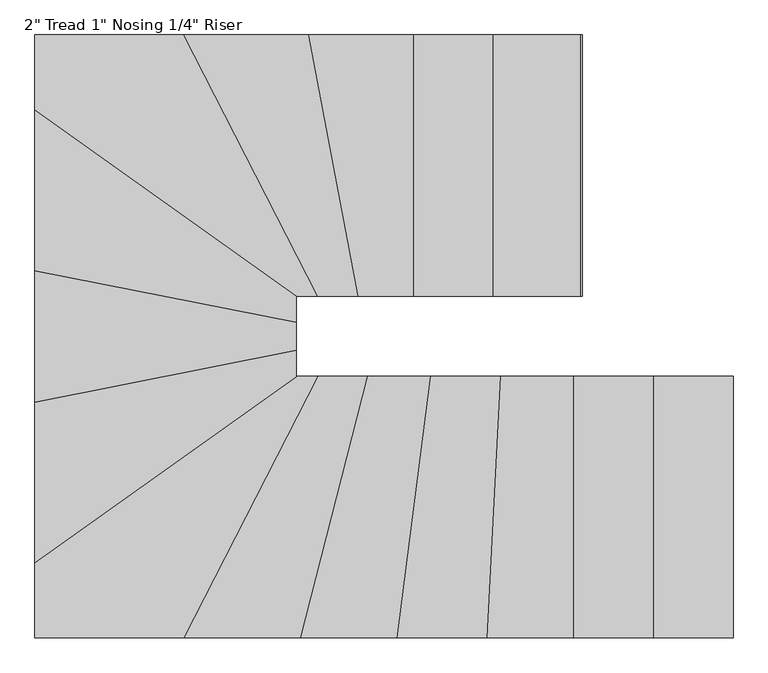
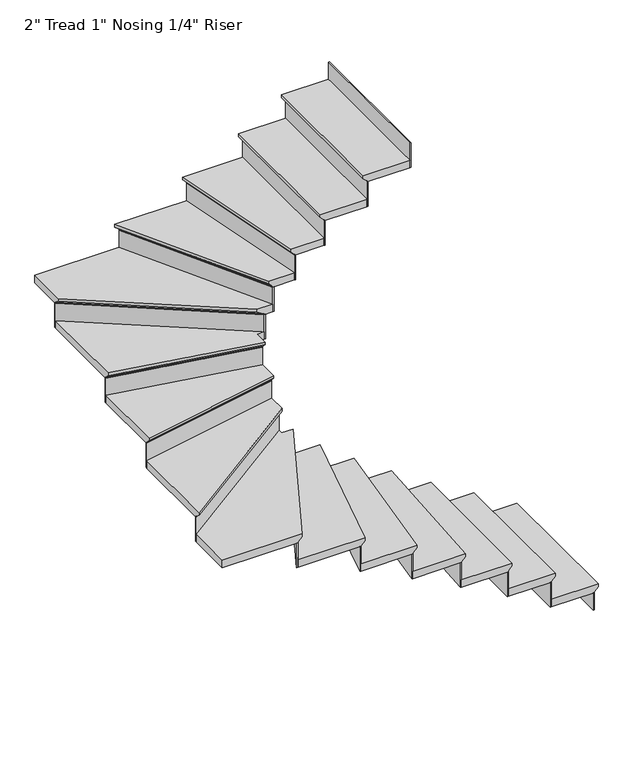
"""IFC4 building model written with IfcOpenShell, lengths in millimetres: stair flight geometry."""

from ifc_helpers import new_model, si_unit, origin, place, context, project, spatial, faceted_brep, source, transform, mapped, element, save


def stair_flight_6de66a2c(model_context):
    return source(origin(), model_context, "Body", "Brep", [
        faceted_brep([(-9238.1085535, 6567.4116886, 150.2833333), (-9238.1085535, 6567.4116886, 169.3333333), (-9238.1085535, 5653.0116886, 169.3333333), (-9238.1085535, 5653.0116886, 150.2833333), (-9263.5085535, 6567.4116886, 124.8833333), (-9263.5085535, 5653.0116886, 124.8833333), (-9542.9085535, 6567.4116886, 169.3333333), (-9542.9085535, 5653.0116886, 169.3333333), (-9263.5085535, 5653.0116886, 118.5333333), (-9542.9085535, 5653.0116886, 118.5333333), (-9542.9085535, 6567.4116886, 118.5333333), (-9263.5085535, 6567.4116886, 118.5333333)], [[[0, 1, 2, 3]], [[4, 0, 3, 5]], [[2, 1, 6, 7]], [[8, 9, 10, 11]], [[2, 7, 9, 8, 5, 3]], [[8, 11, 4, 5]], [[6, 1, 0, 4, 11, 10]], [[7, 6, 10, 9]]]),
        faceted_brep([(-9263.5085535, 6567.4116886, 118.5333333), (-9263.5085535, 6567.4116886, 0.0), (-9269.8585535, 6567.4116886, 0.0), (-9269.8585535, 6567.4116886, 118.5333333), (-9263.5085535, 5653.0116886, 118.5333333), (-9269.8585535, 5653.0116886, 118.5333333), (-9269.8585535, 5653.0116886, 0.0), (-9263.5085535, 5653.0116886, 0.0)], [[[0, 1, 2, 3]], [[4, 5, 6, 7]], [[1, 0, 4, 7]], [[2, 1, 7, 6]], [[3, 2, 6, 5]], [[0, 3, 5, 4]]]),
        faceted_brep([(-9542.9085535, 6567.4116886, 287.8666667), (-9542.9085535, 6567.4116886, 118.5333333), (-9549.2585535, 6567.4116886, 118.5333333), (-9549.2585535, 6567.4116886, 287.8666667), (-9542.9085535, 5653.0116886, 287.8666667), (-9549.2585535, 5653.0116886, 287.8666667), (-9549.2585535, 5653.0116886, 118.5333333), (-9542.9085535, 5653.0116886, 118.5333333)], [[[0, 1, 2, 3]], [[4, 5, 6, 7]], [[1, 0, 4, 7]], [[2, 1, 7, 6]], [[3, 2, 6, 5]], [[0, 3, 5, 4]]]),
        faceted_brep([(-9517.5085535, 5653.0116886, 338.6666667), (-9517.5085535, 6567.4116886, 338.6666667), (-9822.3085535, 6567.4116886, 338.6666667), (-9822.3085535, 5653.0116886, 338.6666667), (-9542.9085535, 5653.0116886, 287.8666667), (-9822.3085535, 5653.0116886, 287.8666667), (-9822.3085535, 6567.4116886, 287.8666667), (-9542.9085535, 6567.4116886, 287.8666667), (-9542.9085535, 5653.0116886, 294.2166667), (-9517.5085535, 5653.0116886, 319.6166667), (-9542.9085535, 6567.4116886, 294.2166667), (-9517.5085535, 6567.4116886, 319.6166667)], [[[0, 1, 2, 3]], [[4, 5, 6, 7]], [[0, 3, 5, 4, 8, 9]], [[4, 7, 10, 8]], [[2, 1, 11, 10, 7, 6]], [[3, 2, 6, 5]], [[11, 1, 0, 9]], [[10, 11, 9, 8]]]),
        faceted_brep([(-9822.3085535, 6567.4116886, 457.2), (-9822.3085535, 6567.4116886, 287.8666667), (-9828.6585535, 6567.4116886, 287.8666667), (-9828.6585535, 6567.4116886, 457.2), (-9822.3085535, 5653.0116886, 457.2), (-9828.6585535, 5653.0116886, 457.2), (-9828.6585535, 5653.0116886, 287.8666667), (-9822.3085535, 5653.0116886, 287.8666667)], [[[0, 1, 2, 3]], [[4, 5, 6, 7]], [[1, 0, 4, 7]], [[2, 1, 7, 6]], [[3, 2, 6, 5]], [[0, 3, 5, 4]]]),
        faceted_brep([(-9796.9085535, 5653.0116886, 508.0), (-9796.9085535, 6567.4116886, 508.0), (-10077.9757149, 6567.4116886, 508.0), (-10125.5099853, 5653.0116886, 508.0), (-9822.3085535, 5653.0116886, 457.2), (-10125.5099853, 5653.0116886, 457.2), (-10077.9757149, 6567.4116886, 457.2), (-9822.3085535, 6567.4116886, 457.2), (-9822.3085535, 5653.0116886, 463.55), (-9796.9085535, 5653.0116886, 488.95), (-9822.3085535, 6567.4116886, 463.55), (-9796.9085535, 6567.4116886, 488.95)], [[[0, 1, 2, 3]], [[4, 5, 6, 7]], [[0, 3, 5, 4, 8, 9]], [[4, 7, 10, 8]], [[2, 1, 11, 10, 7, 6]], [[3, 2, 6, 5]], [[11, 1, 0, 9]], [[10, 11, 9, 8]]]),
        faceted_brep([(-10077.9757149, 6567.4116886, 626.5333333), (-10077.9757149, 6567.4116886, 457.2), (-10084.3342891, 6567.4116886, 457.2), (-10084.3342891, 6567.4116886, 626.5333333), (-10125.5099853, 5653.0116886, 626.5333333), (-10131.8685595, 5653.0116886, 626.5333333), (-10131.8685595, 5653.0116886, 457.2), (-10125.5099853, 5653.0116886, 457.2)], [[[0, 1, 2, 3]], [[4, 5, 6, 7]], [[1, 0, 4, 7]], [[2, 1, 7, 6]], [[3, 2, 6, 5]], [[0, 3, 5, 4]]]),
        faceted_brep([(-10100.0756887, 5653.0116886, 677.3333333), (-10052.5414183, 6567.4116886, 677.3333333), (-10322.1424147, 6567.4116886, 677.3333333), (-10440.4984664, 5653.0116886, 677.3333333), (-10125.5099853, 5653.0116886, 626.5333333), (-10440.4984664, 5653.0116886, 626.5333333), (-10322.1424147, 6567.4116886, 626.5333333), (-10077.9757149, 6567.4116886, 626.5333333), (-10125.5099853, 5653.0116886, 632.8833333), (-10100.0756887, 5653.0116886, 658.2833333), (-10077.9757149, 6567.4116886, 632.8833333), (-10052.5414183, 6567.4116886, 658.2833333)], [[[0, 1, 2, 3]], [[4, 5, 6, 7]], [[0, 3, 5, 4, 8, 9]], [[4, 7, 10, 8]], [[2, 1, 11, 10, 7, 6]], [[3, 2, 6, 5]], [[11, 1, 0, 9]], [[10, 11, 9, 8]]]),
        faceted_brep([(-10322.1424147, 6567.4116886, 795.8666667), (-10322.1424147, 6567.4116886, 626.5333333), (-10328.5453865, 6567.4116886, 626.5333333), (-10328.5453865, 6567.4116886, 795.8666667), (-10440.4984664, 5653.0116886, 795.8666667), (-10446.9014382, 5653.0116886, 795.8666667), (-10446.9014382, 5653.0116886, 626.5333333), (-10440.4984664, 5653.0116886, 626.5333333)], [[[0, 1, 2, 3]], [[4, 5, 6, 7]], [[1, 0, 4, 7]], [[2, 1, 7, 6]], [[3, 2, 6, 5]], [[0, 3, 5, 4]]]),
        faceted_brep([(-10414.8865793, 5653.0116886, 846.6666667), (-10296.5305276, 6567.4116886, 846.6666667), (-10543.7696372, 6567.4116886, 846.6666667), (-10778.9000846, 5653.0116886, 846.6666667), (-10440.4984664, 5653.0116886, 795.8666667), (-10778.9000846, 5653.0116886, 795.8666667), (-10543.7696372, 6567.4116886, 795.8666667), (-10322.1424147, 6567.4116886, 795.8666667), (-10440.4984664, 5653.0116886, 802.2166667), (-10414.8865793, 5653.0116886, 827.6166667), (-10322.1424147, 6567.4116886, 802.2166667), (-10296.5305276, 6567.4116886, 827.6166667)], [[[0, 1, 2, 3]], [[4, 5, 6, 7]], [[0, 3, 5, 4, 8, 9]], [[4, 7, 10, 8]], [[2, 1, 11, 10, 7, 6]], [[3, 2, 6, 5]], [[11, 1, 0, 9]], [[10, 11, 9, 8]]]),
        faceted_brep([(-10543.7696372, 6567.4116886, 965.2), (-10543.7696372, 6567.4116886, 795.8666667), (-10550.3262141, 6567.4116886, 795.8666667), (-10550.3262141, 6567.4116886, 965.2), (-10778.9000846, 5653.0116886, 965.2), (-10785.4566615, 5653.0116886, 965.2), (-10785.4566615, 5653.0116886, 795.8666667), (-10778.9000846, 5653.0116886, 795.8666667)], [[[0, 1, 2, 3]], [[4, 5, 6, 7]], [[1, 0, 4, 7]], [[2, 1, 7, 6]], [[3, 2, 6, 5]], [[0, 3, 5, 4]]]),
        faceted_brep([(-10752.6737772, 5653.0116886, 1016.0), (-10517.5433298, 6567.4116886, 1016.0), (-10720.1162733, 6567.4116886, 1016.0), (-11188.9408946, 5653.0116886, 1016.0), (-10778.9000846, 5653.0116886, 965.2), (-11188.9408946, 5653.0116886, 965.2), (-10720.1162733, 6567.4116886, 965.2), (-10543.7696372, 6567.4116886, 965.2), (-10778.9000846, 5653.0116886, 971.55), (-10752.6737772, 5653.0116886, 996.95), (-10543.7696372, 6567.4116886, 971.55), (-10517.5433298, 6567.4116886, 996.95)], [[[0, 1, 2, 3]], [[4, 5, 6, 7]], [[0, 3, 5, 4, 8, 9]], [[4, 7, 10, 8]], [[2, 1, 11, 10, 7, 6]], [[3, 2, 6, 5]], [[11, 1, 0, 9]], [[10, 11, 9, 8]]]),
        faceted_brep([(-10720.1162733, 6567.4116886, 1134.5333333), (-10720.1162733, 6567.4116886, 965.2), (-10727.2522564, 6567.4116886, 965.2), (-10727.2522564, 6567.4116886, 1134.5333333), (-11188.9408946, 5653.0116886, 1134.5333333), (-11196.0768778, 5653.0116886, 1134.5333333), (-11196.0768778, 5653.0116886, 965.2), (-11188.9408946, 5653.0116886, 965.2)], [[[0, 1, 2, 3]], [[4, 5, 6, 7]], [[1, 0, 4, 7]], [[2, 1, 7, 6]], [[3, 2, 6, 5]], [[0, 3, 5, 4]]]),
        faceted_brep([(-11680.2402453, 5946.6928223, 1185.3333333), (-11680.2402453, 5653.0116886, 1185.3333333), (-11160.3969621, 5653.0116886, 1185.3333333), (-10691.5723408, 6567.4116886, 1185.3333333), (-10765.8402453, 6567.4116886, 1185.3333333), (-10765.8402453, 6596.9667715, 1185.3333333), (-11680.2402453, 5653.0116886, 1134.5333333), (-11680.2402453, 5946.6928223, 1134.5333333), (-10765.8402453, 6596.9667715, 1134.5333333), (-10765.8402453, 6567.4116886, 1134.5333333), (-10720.1162733, 6567.4116886, 1134.5333333), (-11188.9408946, 5653.0116886, 1134.5333333), (-11188.9408946, 5653.0116886, 1140.8833333), (-11160.3969621, 5653.0116886, 1166.2833333), (-10720.1162733, 6567.4116886, 1140.8833333), (-10691.5723408, 6567.4116886, 1166.2833333)], [[[0, 1, 2, 3, 4, 5]], [[6, 7, 8, 9, 10, 11]], [[1, 0, 7, 6]], [[2, 1, 6, 11, 12, 13]], [[11, 10, 14, 12]], [[4, 3, 15, 14, 10, 9]], [[5, 4, 9, 8]], [[0, 5, 8, 7]], [[15, 3, 2, 13]], [[14, 15, 13, 12]]]),
        faceted_brep([(-10765.8402453, 6596.9667715, 1303.8666667), (-10765.8402453, 6596.9667715, 1134.5333333), (-10765.8402453, 6604.7587463, 1134.5333333), (-10765.8402453, 6604.7587463, 1303.8666667), (-11680.2402453, 5946.6928223, 1303.8666667), (-11680.2402453, 5954.4847971, 1303.8666667), (-11680.2402453, 5954.4847971, 1134.5333333), (-11680.2402453, 5946.6928223, 1134.5333333)], [[[0, 1, 2, 3]], [[4, 5, 6, 7]], [[1, 0, 4, 7]], [[2, 1, 7, 6]], [[3, 2, 6, 5]], [[0, 3, 5, 4]]]),
        faceted_brep([(-11680.2402453, 5915.5249231, 1354.6666667), (-10765.8402453, 6565.7988723, 1354.6666667), (-10765.8402453, 6683.4208585, 1354.6666667), (-11680.2402453, 6503.1800022, 1354.6666667), (-11680.2402453, 5946.6928223, 1303.8666667), (-11680.2402453, 6503.1800022, 1303.8666667), (-10765.8402453, 6683.4208585, 1303.8666667), (-10765.8402453, 6596.9667715, 1303.8666667), (-11680.2402453, 5946.6928223, 1310.2166667), (-11680.2402453, 5915.5249231, 1335.6166667), (-10765.8402453, 6596.9667715, 1310.2166667), (-10765.8402453, 6565.7988723, 1335.6166667)], [[[0, 1, 2, 3]], [[4, 5, 6, 7]], [[0, 3, 5, 4, 8, 9]], [[4, 7, 10, 8]], [[2, 1, 11, 10, 7, 6]], [[3, 2, 6, 5]], [[11, 1, 0, 9]], [[10, 11, 9, 8]]]),
        faceted_brep([(-10765.8402453, 6683.4208585, 1473.2), (-10765.8402453, 6683.4208585, 1303.8666667), (-10765.8402453, 6689.893044, 1303.8666667), (-10765.8402453, 6689.893044, 1473.2), (-11680.2402453, 6503.1800022, 1473.2), (-11680.2402453, 6509.6521876, 1473.2), (-11680.2402453, 6509.6521876, 1303.8666667), (-11680.2402453, 6503.1800022, 1303.8666667)], [[[0, 1, 2, 3]], [[4, 5, 6, 7]], [[1, 0, 4, 7]], [[2, 1, 7, 6]], [[3, 2, 6, 5]], [[0, 3, 5, 4]]]),
        faceted_brep([(-11680.2402453, 6477.2912605, 1524.0), (-10765.8402453, 6657.5321168, 1524.0), (-10765.8402453, 6782.5800022, 1524.0), (-11680.2402453, 6962.8208585, 1524.0), (-11680.2402453, 6503.1800022, 1473.2), (-11680.2402453, 6962.8208585, 1473.2), (-10765.8402453, 6782.5800022, 1473.2), (-10765.8402453, 6683.4208585, 1473.2), (-11680.2402453, 6503.1800022, 1479.55), (-11680.2402453, 6477.2912605, 1504.95), (-10765.8402453, 6683.4208585, 1479.55), (-10765.8402453, 6657.5321168, 1504.95)], [[[0, 1, 2, 3]], [[4, 5, 6, 7]], [[0, 3, 5, 4, 8, 9]], [[4, 7, 10, 8]], [[2, 1, 11, 10, 7, 6]], [[3, 2, 6, 5]], [[11, 1, 0, 9]], [[10, 11, 9, 8]]]),
        faceted_brep([(-10765.8402453, 6782.5800022, 1642.5333333), (-10765.8402453, 6782.5800022, 1473.2), (-10765.8402453, 6789.0521876, 1473.2), (-10765.8402453, 6789.0521876, 1642.5333333), (-11680.2402453, 6962.8208585, 1642.5333333), (-11680.2402453, 6969.293044, 1642.5333333), (-11680.2402453, 6969.293044, 1473.2), (-11680.2402453, 6962.8208585, 1473.2)], [[[0, 1, 2, 3]], [[4, 5, 6, 7]], [[1, 0, 4, 7]], [[2, 1, 7, 6]], [[3, 2, 6, 5]], [[0, 3, 5, 4]]]),
        faceted_brep([(-11680.2402453, 6936.9321168, 1693.3333333), (-10765.8402453, 6756.6912605, 1693.3333333), (-10765.8402453, 6846.8116886, 1693.3333333), (-10719.7447708, 6846.8116886, 1693.3333333), (-11680.2402453, 7529.8663533, 1693.3333333), (-11680.2402453, 6962.8208585, 1642.5333333), (-11680.2402453, 7529.8663533, 1642.5333333), (-10719.7447708, 6846.8116886, 1642.5333333), (-10765.8402453, 6846.8116886, 1642.5333333), (-10765.8402453, 6782.5800022, 1642.5333333), (-11680.2402453, 6962.8208585, 1648.8833333), (-11680.2402453, 6936.9321168, 1674.2833333), (-10765.8402453, 6782.5800022, 1648.8833333), (-10765.8402453, 6756.6912605, 1674.2833333)], [[[0, 1, 2, 3, 4]], [[5, 6, 7, 8, 9]], [[0, 4, 6, 5, 10, 11]], [[5, 9, 12, 10]], [[2, 1, 13, 12, 9, 8]], [[3, 2, 8, 7]], [[4, 3, 7, 6]], [[13, 1, 0, 11]], [[12, 13, 11, 10]]]),
        faceted_brep([(-10719.7447708, 6846.8116886, 1811.8666667), (-10719.7447708, 6846.8116886, 1642.5333333), (-10708.7878783, 6846.8116886, 1642.5333333), (-10708.7878783, 6846.8116886, 1811.8666667), (-11680.2402453, 7529.8663533, 1811.8666667), (-11680.2402453, 7537.6583281, 1811.8666667), (-11680.2402453, 7537.6583281, 1642.5333333), (-11680.2402453, 7529.8663533, 1642.5333333)], [[[0, 1, 2, 3]], [[4, 5, 6, 7]], [[1, 0, 4, 7]], [[2, 1, 7, 6]], [[3, 2, 6, 5]], [[0, 3, 5, 4]]]),
        faceted_brep([(-11131.8530296, 7761.2116886, 1862.6666667), (-11680.2402453, 7761.2116886, 1862.6666667), (-11680.2402453, 7498.6984541, 1862.6666667), (-10763.5723408, 6846.8116886, 1862.6666667), (-10663.0284082, 6846.8116886, 1862.6666667), (-11680.2402453, 7761.2116886, 1811.8666667), (-11131.8530296, 7761.2116886, 1811.8666667), (-10663.0284082, 6846.8116886, 1811.8666667), (-10719.7447708, 6846.8116886, 1811.8666667), (-11680.2402453, 7529.8663533, 1811.8666667), (-11680.2402453, 7529.8663533, 1818.2166667), (-11680.2402453, 7498.6984541, 1843.6166667), (-10719.7447708, 6846.8116886, 1818.2166667), (-10763.5723408, 6846.8116886, 1843.6166667)], [[[0, 1, 2, 3, 4]], [[5, 6, 7, 8, 9]], [[1, 0, 6, 5]], [[2, 1, 5, 9, 10, 11]], [[9, 8, 12, 10]], [[4, 3, 13, 12, 8, 7]], [[0, 4, 7, 6]], [[13, 3, 2, 11]], [[12, 13, 11, 10]]]),
        faceted_brep([(-10663.0284082, 6846.8116886, 1981.2), (-10663.0284082, 6846.8116886, 1811.8666667), (-10655.8924251, 6846.8116886, 1811.8666667), (-10655.8924251, 6846.8116886, 1981.2), (-11131.8530296, 7761.2116886, 1981.2), (-11124.7170464, 7761.2116886, 1981.2), (-11124.7170464, 7761.2116886, 1811.8666667), (-11131.8530296, 7761.2116886, 1811.8666667)], [[[0, 1, 2, 3]], [[4, 5, 6, 7]], [[1, 0, 4, 7]], [[2, 1, 7, 6]], [[3, 2, 6, 5]], [[0, 3, 5, 4]]]),
        faceted_brep([(-11160.3969621, 7761.2116886, 2032.0), (-10691.5723408, 6846.8116886, 2032.0), (-10522.7881155, 6846.8116886, 2032.0), (-10695.7284139, 7761.2116886, 2032.0), (-11131.8530296, 7761.2116886, 1981.2), (-10695.7284139, 7761.2116886, 1981.2), (-10522.7881155, 6846.8116886, 1981.2), (-10663.0284082, 6846.8116886, 1981.2), (-11131.8530296, 7761.2116886, 1987.55), (-11160.3969621, 7761.2116886, 2012.95), (-10663.0284082, 6846.8116886, 1987.55), (-10691.5723408, 6846.8116886, 2012.95)], [[[0, 1, 2, 3]], [[4, 5, 6, 7]], [[0, 3, 5, 4, 8, 9]], [[4, 7, 10, 8]], [[2, 1, 11, 10, 7, 6]], [[3, 2, 6, 5]], [[11, 1, 0, 9]], [[10, 11, 9, 8]]]),
        faceted_brep([(-10522.7881155, 6846.8116886, 2150.5333333), (-10522.7881155, 6846.8116886, 1981.2), (-10516.3255434, 6846.8116886, 1981.2), (-10516.3255434, 6846.8116886, 2150.5333333), (-10695.7284139, 7761.2116886, 2150.5333333), (-10689.2658417, 7761.2116886, 2150.5333333), (-10689.2658417, 7761.2116886, 1981.2), (-10695.7284139, 7761.2116886, 1981.2)], [[[0, 1, 2, 3]], [[4, 5, 6, 7]], [[1, 0, 4, 7]], [[2, 1, 7, 6]], [[3, 2, 6, 5]], [[0, 3, 5, 4]]]),
        faceted_brep([(-10721.5787026, 7761.2116886, 2201.3333333), (-10548.6384043, 6846.8116886, 2201.3333333), (-10330.3085535, 6846.8116886, 2201.3333333), (-10330.3085535, 7761.2116886, 2201.3333333), (-10695.7284139, 7761.2116886, 2150.5333333), (-10330.3085535, 7761.2116886, 2150.5333333), (-10330.3085535, 6846.8116886, 2150.5333333), (-10522.7881155, 6846.8116886, 2150.5333333), (-10695.7284139, 7761.2116886, 2156.8833333), (-10721.5787026, 7761.2116886, 2182.2833333), (-10522.7881155, 6846.8116886, 2156.8833333), (-10548.6384043, 6846.8116886, 2182.2833333)], [[[0, 1, 2, 3]], [[4, 5, 6, 7]], [[0, 3, 5, 4, 8, 9]], [[4, 7, 10, 8]], [[2, 1, 11, 10, 7, 6]], [[3, 2, 6, 5]], [[11, 1, 0, 9]], [[10, 11, 9, 8]]]),
        faceted_brep([(-10330.3085535, 6846.8116886, 2319.8666667), (-10330.3085535, 6846.8116886, 2150.5333333), (-10323.9585535, 6846.8116886, 2150.5333333), (-10323.9585535, 6846.8116886, 2319.8666667), (-10330.3085535, 7761.2116886, 2319.8666667), (-10323.9585535, 7761.2116886, 2319.8666667), (-10323.9585535, 7761.2116886, 2150.5333333), (-10330.3085535, 7761.2116886, 2150.5333333)], [[[0, 1, 2, 3]], [[4, 5, 6, 7]], [[1, 0, 4, 7]], [[2, 1, 7, 6]], [[3, 2, 6, 5]], [[0, 3, 5, 4]]]),
        faceted_brep([(-10355.7085535, 7761.2116886, 2370.6666667), (-10355.7085535, 6846.8116886, 2370.6666667), (-10050.9085535, 6846.8116886, 2370.6666667), (-10050.9085535, 7761.2116886, 2370.6666667), (-10330.3085535, 7761.2116886, 2319.8666667), (-10050.9085535, 7761.2116886, 2319.8666667), (-10050.9085535, 6846.8116886, 2319.8666667), (-10330.3085535, 6846.8116886, 2319.8666667), (-10330.3085535, 7761.2116886, 2326.2166667), (-10355.7085535, 7761.2116886, 2351.6166667), (-10330.3085535, 6846.8116886, 2326.2166667), (-10355.7085535, 6846.8116886, 2351.6166667)], [[[0, 1, 2, 3]], [[4, 5, 6, 7]], [[0, 3, 5, 4, 8, 9]], [[4, 7, 10, 8]], [[2, 1, 11, 10, 7, 6]], [[3, 2, 6, 5]], [[11, 1, 0, 9]], [[10, 11, 9, 8]]]),
        faceted_brep([(-10050.9085535, 6846.8116886, 2489.2), (-10050.9085535, 6846.8116886, 2319.8666667), (-10044.5585535, 6846.8116886, 2319.8666667), (-10044.5585535, 6846.8116886, 2489.2), (-10050.9085535, 7761.2116886, 2489.2), (-10044.5585535, 7761.2116886, 2489.2), (-10044.5585535, 7761.2116886, 2319.8666667), (-10050.9085535, 7761.2116886, 2319.8666667)], [[[0, 1, 2, 3]], [[4, 5, 6, 7]], [[1, 0, 4, 7]], [[2, 1, 7, 6]], [[3, 2, 6, 5]], [[0, 3, 5, 4]]]),
        faceted_brep([(-9771.5085535, 6846.8116886, 2658.5333333), (-9771.5085535, 6846.8116886, 2489.2), (-9765.1585535, 6846.8116886, 2489.2), (-9765.1585535, 6846.8116886, 2658.5333333), (-9771.5085535, 7761.2116886, 2658.5333333), (-9765.1585535, 7761.2116886, 2658.5333333), (-9765.1585535, 7761.2116886, 2489.2), (-9771.5085535, 7761.2116886, 2489.2)], [[[0, 1, 2, 3]], [[4, 5, 6, 7]], [[1, 0, 4, 7]], [[2, 1, 7, 6]], [[3, 2, 6, 5]], [[0, 3, 5, 4]]]),
        faceted_brep([(-10076.3085535, 7761.2116886, 2540.0), (-10076.3085535, 6846.8116886, 2540.0), (-9771.5085535, 6846.8116886, 2540.0), (-9771.5085535, 7761.2116886, 2540.0), (-10050.9085535, 7761.2116886, 2489.2), (-9771.5085535, 7761.2116886, 2489.2), (-9771.5085535, 6846.8116886, 2489.2), (-10050.9085535, 6846.8116886, 2489.2), (-10050.9085535, 7761.2116886, 2495.55), (-10076.3085535, 7761.2116886, 2520.95), (-10050.9085535, 6846.8116886, 2495.55), (-10076.3085535, 6846.8116886, 2520.95)], [[[0, 1, 2, 3]], [[4, 5, 6, 7]], [[0, 3, 5, 4, 8, 9]], [[4, 7, 10, 8]], [[2, 1, 11, 10, 7, 6]], [[3, 2, 6, 5]], [[11, 1, 0, 9]], [[10, 11, 9, 8]]]),
    ])


if __name__ == "__main__":
    model = new_model("IFC4")
    model_context = context("Model", 3, world=origin())
    ifc_project = project(units=[si_unit("LENGTHUNIT", "METRE", prefix="MILLI")], contexts=[model_context])
    site = spatial("IfcSite", under=ifc_project)
    building = spatial("IfcBuilding", under=site)
    placement = place(None, origin())
    stair_flight_shape = stair_flight_6de66a2c(model_context)
    element("IfcStairFlight", 1, ObjectType="2\" Tread 1\" Nosing 1/4\" Riser", at=placement, inside=building, context=model_context, shape_type="MappedRepresentation", body=[
        mapped(stair_flight_shape, transform((0.0, 0.0, 0.0), x_axis=(1.0, 0.0, 0.0), y_axis=(0.0, 1.0, 0.0), z_axis=(0.0, 0.0, 1.0))),
    ])
    save(model, "model.ifc")
